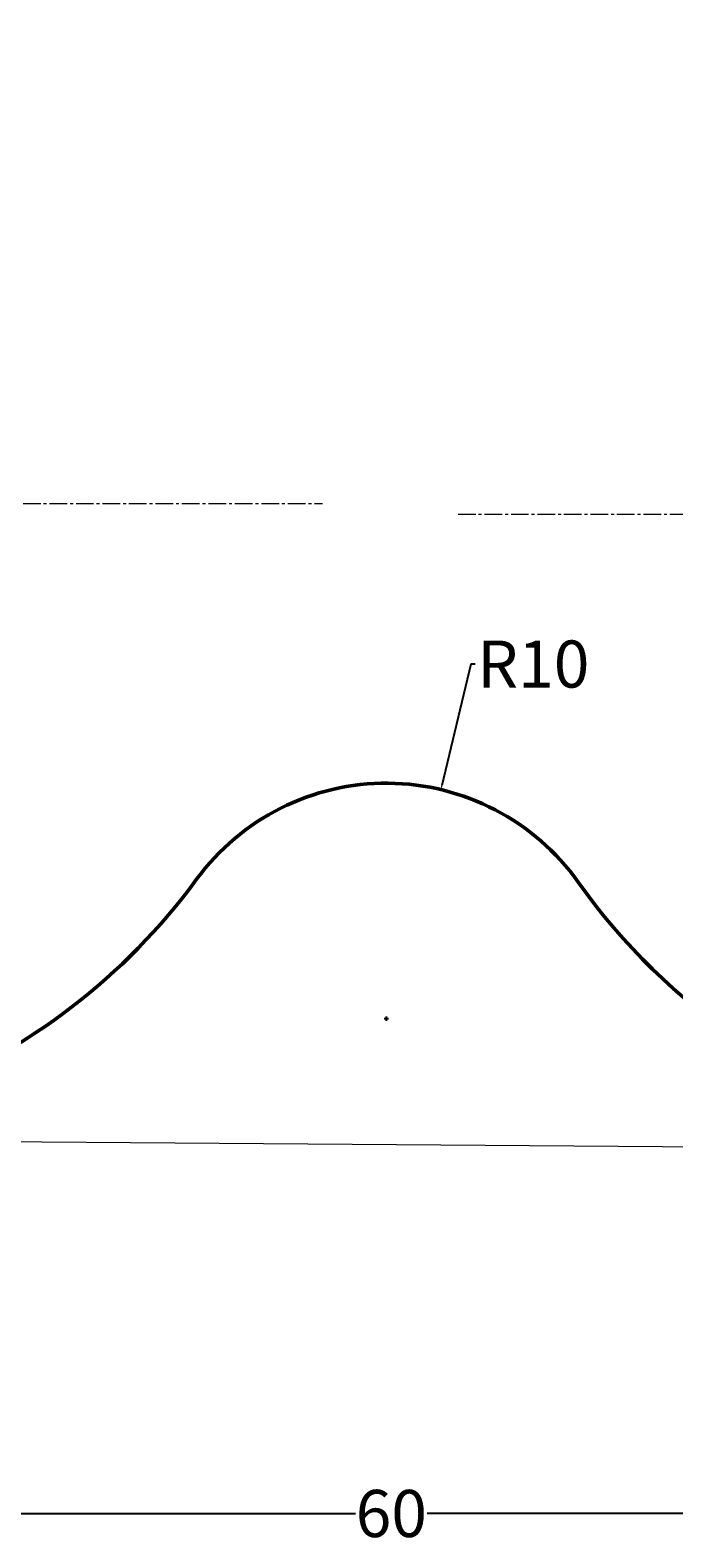
# Model space of a CAD drawing. Units: millimetres. Extents: x -60 to 113, y -37 to 126.
# Tile 5 of 17: x 22 to 49, y -37 to 27. Entities that reach past the tile are written whole.
import ezdxf

# ---------------------------------------------------------------- set-up
doc = ezdxf.new("R2010")
doc.units = ezdxf.units.MM
doc.header["$MEASUREMENT"] = 0
doc.linetypes.add('CENTER2', pattern=[1.125, 0.75, -0.125, 0.125, -0.125])
for name, color, linetype, lineweight in [('M-CNTR', 4, 'CENTER2', 18), ('M-CONS', 8, 'Continuous', 13), ('M-DIMS', 2, 'Continuous', 25), ('M-OUTL', 7, 'Continuous', 50)]:
    doc.layers.add(name, color=color, linetype=linetype, lineweight=lineweight)
doc.styles.get("Standard").update_dxf_attribs({"font": 'arial.ttf'})
doc.dimstyles.get("Standard").update_dxf_attribs({"dimtxt": 0.18, "dimasz": 0.18, "dimexe": 0.18, "dimexo": 0.0625, "dimgap": 0.09, "dimtad": 0, "dimtih": 1, "dimtoh": 1, "dimdec": 4, "dimzin": 0, "dimdsep": 46, "dimtxsty": 'Standard', "dimcen": 0.09, "dimadec": 0, "dimazin": 0, "dimtfac": 1, "dimtdec": 4, "dimtofl": 0, "dimtmove": 0, "dimatfit": 3, "dimfxl": 1, "dimtolj": 1, "dimtzin": 0, "dimarcsym": 0})

# ---------------------------------------------------------------- blocks, each defined once
blk = doc.blocks.new('*U2')
at = {"layer": 'M-CNTR', "color": 0, "transparency": 16777216}
for p, q in [((0, 5.4), (0, 27.12)), ((-27.12, 0), (-5.4, 0)), ((5.4, 0), (27.12, 0)), ((0, -27.12), (0, -5.4))]:
    blk.add_line(p, q, dxfattribs=at)
at = {"layer": 'M-CNTR', "color": 0, "linetype": 'Continuous', "transparency": 16777216}
for p, q in [((0, -2.7), (0, 2.7)), ((-2.7, 0), (2.7, 0))]:
    blk.add_line(p, q, dxfattribs=at)
blk = doc.blocks.new('*U3')
at = {"layer": 'M-CNTR', "color": 0, "transparency": 16777216}
for p, q in [((0, 5.4), (0, 27.12)), ((-27.12, 0), (-5.4, 0)), ((5.4, 0), (27.12, 0)), ((0, -27.12), (0, -5.4))]:
    blk.add_line(p, q, dxfattribs=at)
at = {"layer": 'M-CNTR', "color": 0, "linetype": 'Continuous', "transparency": 16777216}
for p, q in [((0, -2.7), (0, 2.7)), ((-2.7, 0), (2.7, 0))]:
    blk.add_line(p, q, dxfattribs=at)
blk = doc.blocks.new('*D10')
at = {"layer": 'Defpoints', "color": 0, "transparency": 16777216}
for p in [(39.417, -5.256), (37.099, -14.984)]:
    blk.add_point(p, dxfattribs=at)
at = {"layer": 'M-DIMS', "color": 0, "lineweight": -2, "transparency": 16777216}
for p, q in [((40.688, 0.078), (39.459, -5.081)), ((40.868, 0.078), (40.688, 0.078)), ((37.009, -14.984), (37.189, -14.984)), ((37.099, -15.074), (37.099, -14.894))]:
    blk.add_line(p, q, dxfattribs=at)
at = {"layer": 'M-DIMS', "color": 0, "transparency": 16777216}
blk.add_solid([(39.43, -5.074), (39.488, -5.088), (39.417, -5.256)], dxfattribs=at)
at = {"layer": 'M-DIMS', "color": 0, "transparency": 16777216, "insert": (43.345, 0.078), "char_height": 0.18, "attachment_point": 5}
blk.add_mtext('\\A1;{\\H11.11111x;R10}', dxfattribs=at)
blk = doc.blocks.new('*D13')
at = {"layer": 'Defpoints', "color": 0, "transparency": 16777216}
for p in [(37.065, 46.813), (-39.303, 6.903), (7.267, 6.903)]:
    blk.add_point(p, dxfattribs=at)
at = {"layer": 'M-DIMS', "color": 0, "lineweight": -2, "transparency": 16777216}
for p, q in [((37.002, 46.813), (-39.483, 46.813)), ((-39.303, 46.633), (-39.303, 27.969)), ((-39.303, 7.083), (-39.303, 25.747)), ((7.204, 6.903), (-39.483, 6.903))]:
    blk.add_line(p, q, dxfattribs=at)
at = {"layer": 'M-DIMS', "color": 0, "transparency": 16777216}
for points in [[(-39.333, 46.633), (-39.273, 46.633), (-39.303, 46.813)], [(-39.333, 7.083), (-39.273, 7.083), (-39.303, 6.903)]]:
    blk.add_solid(points, dxfattribs=at)
at = {"layer": 'M-DIMS', "color": 0, "transparency": 16777216, "insert": (-39.303, 26.858), "char_height": 0.18, "attachment_point": 5}
blk.add_mtext('\\A1;{\\H11.11111x;40}', dxfattribs=at)
blk = doc.blocks.new('*D14')
at = {"layer": 'Defpoints', "color": 0, "transparency": 16777216}
for p in [(7.267, 6.903), (67.355, 6.442), (67.355, -36.011)]:
    blk.add_point(p, dxfattribs=at)
at = {"layer": 'M-DIMS', "color": 0, "lineweight": -2, "transparency": 16777216}
for p, q in [((7.267, 6.84), (7.267, -36.191)), ((67.355, 6.379), (67.355, -36.191)), ((7.447, -36.011), (35.786, -36.011)), ((67.175, -36.011), (38.835, -36.011))]:
    blk.add_line(p, q, dxfattribs=at)
at = {"layer": 'M-DIMS', "color": 0, "transparency": 16777216}
for points in [[(7.447, -35.981), (7.447, -36.041), (7.267, -36.011)], [(67.175, -35.981), (67.175, -36.041), (67.355, -36.011)]]:
    blk.add_solid(points, dxfattribs=at)
at = {"layer": 'M-DIMS', "color": 0, "transparency": 16777216, "insert": (37.311, -36.011), "char_height": 0.18, "attachment_point": 5}
blk.add_mtext('\\A1;{\\H11.11111x;60}', dxfattribs=at)
blk = doc.blocks.new('*D17')
at = {"layer": 'Defpoints', "color": 0, "transparency": 16777216}
for p in [(67.355, 124.823), (10.532, 88.533), (67.355, 6.442)]:
    blk.add_point(p, dxfattribs=at)
at = {"layer": 'M-DIMS', "color": 0, "lineweight": -2, "transparency": 16777216}
for p, q in [((10.532, 88.595), (10.532, 125.003)), ((67.355, 6.504), (67.355, 125.003)), ((10.712, 124.823), (37.422, 124.823)), ((67.175, 124.823), (40.465, 124.823))]:
    blk.add_line(p, q, dxfattribs=at)
at = {"layer": 'M-DIMS', "color": 0, "transparency": 16777216}
for points in [[(10.712, 124.853), (10.712, 124.793), (10.532, 124.823)], [(67.175, 124.853), (67.175, 124.793), (67.355, 124.823)]]:
    blk.add_solid(points, dxfattribs=at)
at = {"layer": 'M-DIMS', "color": 0, "transparency": 16777216, "insert": (38.944, 124.823), "char_height": 0.18, "attachment_point": 5}
blk.add_mtext('\\A1;{\\H11.11111x;56}', dxfattribs=at)

msp = doc.modelspace()

# ---------------------------------------------------------------- linework, layer by layer
at = {"layer": 'M-CONS'}
msp.add_line((7.05918, -20.09651), (67.05741, -20.55741), dxfattribs=at)
at = {"layer": 'M-OUTL'}
for centre, radius, start, end in [((67.26481, 6.44179), 27, 215.3846391, 96.5826838), ((7.26659, 6.9027), 27, 131.8666546, 323.7350904), ((37.09934, -14.98352), 10, 35.3846391, 143.7350904)]:
    msp.add_arc(centre, radius, start, end, dxfattribs=at)

# ---------------------------------------------------------------- block references
at = {"layer": 'M-CNTR'}
for name, p in [('*U2', (7.26659, 6.9027)), ('*U3', (67.26481, 6.44179))]:
    msp.add_blockref(name, p, dxfattribs=at)

# ---------------------------------------------------------------- dimensions: what is measured, and where the dimension line sits
at = {"layer": 'M-DIMS'}
for base, p1, text, picture, middle in [((67.35481, 124.82251), (10.53227, 88.53289), '{\\H11.11111x;56}', '*D17', (38.94354, 124.82251)), ((67.35481, -36.0105), (7.26659, 6.9027), '{\\H11.11111x;60}', '*D14', (37.3107, -36.0105))]:
    dim = msp.add_linear_dim(base=base, p1=p1, p2=(67.35481, 6.44179), text=text, dimstyle='Standard', override={"dimclrd": 0, "dimclre": 0, "dimclrt": 0}, dxfattribs=at)
    dim.commit()
    dim.dimension.update_dxf_attribs({"geometry": picture, "text_midpoint": middle})
dim = msp.add_linear_dim(base=(-39.30316, 6.9027), p1=(37.06463, 46.81263), p2=(7.26659, 6.9027), angle=90, text='{\\H11.11111x;40}', dimstyle='Standard', override={"dimclrd": 0, "dimclre": 0, "dimclrt": 0}, dxfattribs=at)
dim.commit()
dim.dimension.update_dxf_attribs({"geometry": '*D13', "text_midpoint": (-39.30316, 26.85766)})
dim = msp.add_radius_dim(center=(37.09934, -14.98352), mpoint=(39.41741, -5.25591), text='{\\H11.11111x;R10}', dimstyle='Standard', override={"dimclrd": 0, "dimclre": 0, "dimclrt": 0}, dxfattribs=at)
dim.commit()
dim.dimension.update_dxf_attribs({"geometry": '*D10', "text_midpoint": (43.34456, 0.07805), "dimtype": 164})

doc.saveas('drawing.dxf')
